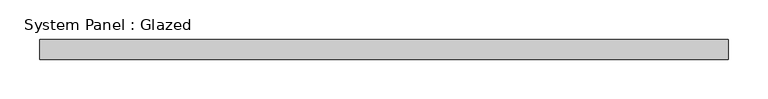
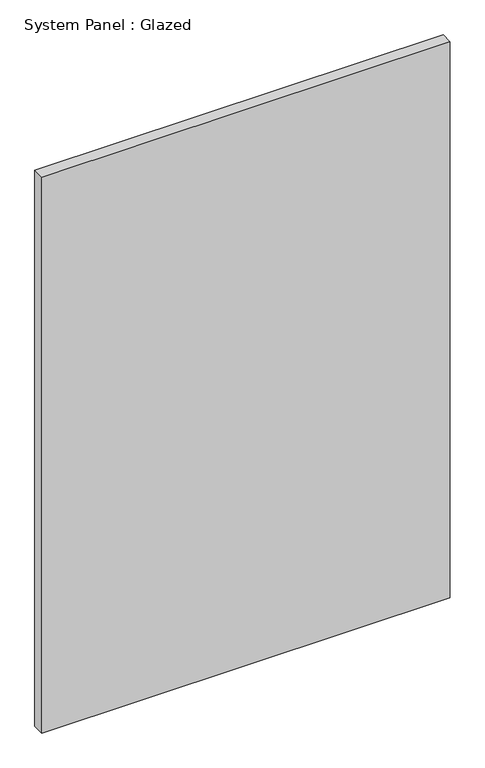
"""IFC4 building model written with IfcOpenShell, lengths in millimetres: plate geometry, System Panel : Glazed."""

from ifc_helpers import new_model, si_unit, origin, origin_with_axes, place, context, project, spatial, polyline, outline, extrude, source, transform, mapped, element, save


def system_panel_glazed_3cfdd687(model_context):
    return source(origin(), model_context, "Body", "SweptSolid", [
        extrude(outline(polyline([(434.975, 19.05), (-434.975, 19.05), (-434.975, 44.45), (434.975, 44.45), (434.975, 19.05)])), origin_with_axes(), (0.0, 0.0, 1.0), 1251.4977008),
    ])


if __name__ == "__main__":
    model = new_model("IFC4")
    model_context = context("Model", 3, world=origin())
    ifc_project = project(units=[si_unit("LENGTHUNIT", "METRE", prefix="MILLI")], contexts=[model_context])
    site = spatial("IfcSite", under=ifc_project)
    building = spatial("IfcBuilding", under=site)
    placement = place(None, origin())
    system_panel_glazed_shape = system_panel_glazed_3cfdd687(model_context)
    element("IfcPlate", 1, ObjectType="System Panel : Glazed", at=placement, inside=building, context=model_context, shape_type="MappedRepresentation", body=[
        mapped(system_panel_glazed_shape, transform((0.0, 0.0, 0.0), x_axis=(1.0, 0.0, 0.0), y_axis=(0.0, 1.0, 0.0), z_axis=(0.0, 0.0, 1.0))),
    ])
    save(model, "model.ifc")

# Revit data of these elements
# Type "System Panel : Glazed"
#   Construction Type Id = "GSP4R"
#   Analytic Construction = "1/8 in Pilkington single glazing"
#   Visual Light Transmittance = 0.9
#   Solar Heat Gain Coefficient = 0.86
#   Heat Transfer Coefficient (U) = 1.18115 BTU/(h·ft²·°F)
#   Define Thermal Properties by = 1
# Element 1 (IfcPlate, "System Panel : Glazed")
#   Materials on its faces: "Glass"
# Materials
#   "Glass": class "Glass", colour RGB 0 128 192, transparency 0.75, Description = "Soda Lime Glass", Cost = 0
